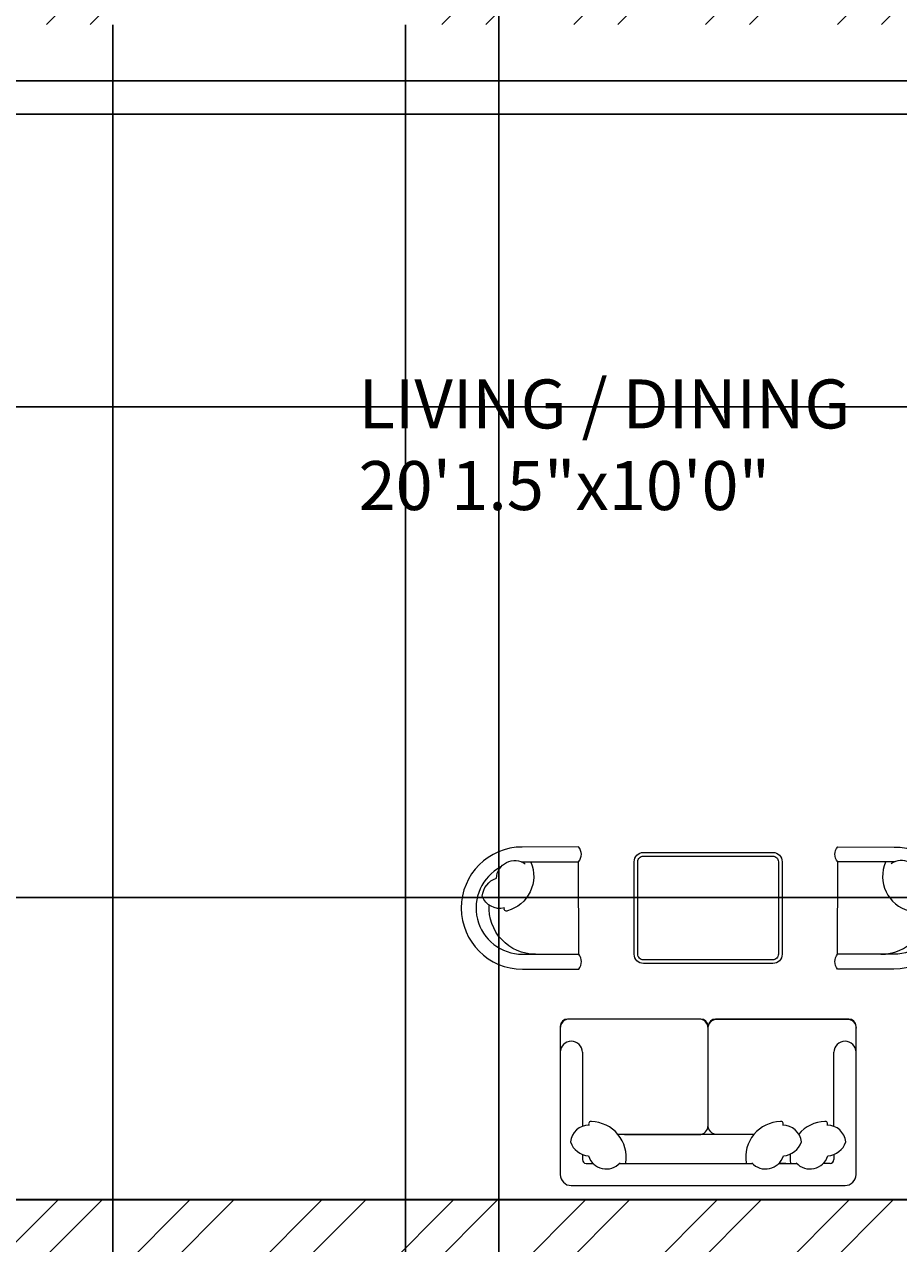
# Model space of a CAD drawing. Units: inches. Extents: x 1748 to 2382, y 1346 to 2284.
# Tile 9 of 26: x 1920 to 2009, y 1730 to 1855. Entities that reach past the tile are written whole.
import ezdxf

# ---------------------------------------------------------------- set-up
doc = ezdxf.new("R2010")
doc.units = ezdxf.units.IN
for name, color, linetype, lineweight in [('A-ANNO-DIMS', 2, 'Continuous', 18), ('A-AREA-IDEN', 7, 'Continuous', 18), ('A-FURN', 8, 'Continuous', 13), ('A-WALL', 7, 'Continuous', 35), ('A-WALL-PATT', 9, 'Continuous', 13)]:
    doc.layers.add(name, color=color, linetype=linetype, lineweight=lineweight)
doc.styles.get("Standard").update_dxf_attribs({"font": 'arial.ttf'})
doc.dimstyles.get("Standard").update_dxf_attribs({"dimtxt": 0.18, "dimasz": 0.18, "dimexe": 0.18, "dimexo": 0.0625, "dimgap": 0.09, "dimtad": 0, "dimtih": 1, "dimtoh": 1, "dimdec": 4, "dimzin": 0, "dimdsep": 46, "dimtxsty": 'Standard', "dimcen": 0.09, "dimadec": 0, "dimazin": 0, "dimtfac": 1, "dimtdec": 4, "dimtofl": 0, "dimtmove": 0, "dimatfit": 3, "dimfxl": 1, "dimtolj": 1, "dimtzin": 0, "dimarcsym": 0})

# ---------------------------------------------------------------- blocks, each defined once
blk = doc.blocks.new('A$C1352')
at = {"color": 0}
for points in [[(0.0027, 0.053), (0.0027, 0.553, -0.414214), (0.0527, 0.603), (0.7527, 0.603, -0.414214), (0.8027, 0.553), (0.8027, 0.053, -0.414214), (0.7527, 0.003), (0.0527, 0.003, -0.414214)], [(0.0227, 0.053), (0.0227, 0.553, -0.414214), (0.0527, 0.583), (0.7527, 0.583, -0.414214), (0.7827, 0.553), (0.7827, 0.053, -0.414214), (0.7527, 0.023), (0.0527, 0.023, -0.414214)]]:
    blk.add_lwpolyline(points, format="xyb", close=True, dxfattribs=at)
blk = doc.blocks.new('CHAIR-LOUNGE')
blk.add_line((1.52, 6.05), (1.51, 0.29))
at = {"ltscale": 0.03}
blk.add_lwpolyline([(1.51, 0.29, -0.369229), (0, 0.29), (0.01, 6.05, -1), (12.48, 6.04), (12.47, 0.28, -0.369229), (10.96, 0.28)], format="xyb", close=True, dxfattribs=at)
blk.add_lwpolyline([(2.05, 8.23, -0.785087), (10.96, 6.04), (10.96, 0.28)], format="xyb")
for centre, radius, start, end in [((5.21, 8.01), 2.13, 94.9999, 161.3534), ((4.35, 8.32), 1.94, 346.6403, 69.4695), ((6.24, 4.71), 4.72, 359.9461, 93.658), ((3.29, 6.8), 1.89, 92.9922, 214.1401), ((3, 8.54), 3.66, 247.0143, 344.2857), ((6.33, 7.66), 0.226, 330.6238, 113.7423), ((6.24, 6.05), 4.72, 178.8536, 179.9461)]:
    blk.add_arc(centre, radius, start, end)
blk = doc.blocks.new('*D48')
at = {"layer": 'A-ANNO-DIMS', "color": 0, "lineweight": -2, "transparency": 16777216}
for p, q in [((2130.9, 1849.07), (1779.88, 1849.07)), ((1780.06, 1848.89), (1780.06, 1832.62)), ((1780.06, 1815.98), (1780.06, 1832.25)), ((2130.9, 1815.8), (1779.88, 1815.8))]:
    blk.add_line(p, q, dxfattribs=at)
at = {"layer": 'A-ANNO-DIMS', "color": 0, "transparency": 16777216}
for points in [[(1780.03, 1848.89), (1780.09, 1848.89), (1780.06, 1849.07)], [(1780.03, 1815.98), (1780.09, 1815.98), (1780.06, 1815.8)]]:
    blk.add_solid(points, dxfattribs=at)
at = {"layer": 'Defpoints', "color": 0, "transparency": 16777216}
for p in [(1780.06, 1849.07), (2130.96, 1849.07), (2130.96, 1815.8)]:
    blk.add_point(p, dxfattribs=at)
at = {"layer": 'A-ANNO-DIMS', "color": 0, "transparency": 16777216, "insert": (1780.06, 1832.43), "char_height": 0.18, "attachment_point": 5}
blk.add_mtext('\\A1;33.27', dxfattribs=at)
blk = doc.blocks.new('*D51')
at = {"layer": 'A-ANNO-DIMS', "color": 0, "lineweight": -2, "transparency": 16777216}
for p, q in [((1968.44, 2223.79), (1968.44, 1360.47)), ((2040.07, 2223.79), (2040.07, 1360.47)), ((1968.62, 1360.65), (2003.86, 1360.65)), ((2039.89, 1360.65), (2004.65, 1360.65))]:
    blk.add_line(p, q, dxfattribs=at)
at = {"layer": 'A-ANNO-DIMS', "color": 0, "transparency": 16777216}
for points in [[(1968.62, 1360.68), (1968.62, 1360.62), (1968.44, 1360.65)], [(2039.89, 1360.68), (2039.89, 1360.62), (2040.07, 1360.65)]]:
    blk.add_solid(points, dxfattribs=at)
at = {"layer": 'Defpoints', "color": 0, "transparency": 16777216}
for p in [(1968.44, 2223.85), (2040.07, 2223.85), (2040.07, 1360.65)]:
    blk.add_point(p, dxfattribs=at)
at = {"layer": 'A-ANNO-DIMS', "color": 0, "transparency": 16777216, "insert": (2004.26, 1360.65), "char_height": 0.18, "attachment_point": 5}
blk.add_mtext('\\A1;71.62', dxfattribs=at)
blk = doc.blocks.new('*D60')
at = {"layer": 'A-ANNO-DIMS', "color": 0, "lineweight": -2, "transparency": 16777216}
for p, q in [((2206.01, 1845.68), (1779.88, 1845.68)), ((1780.06, 1845.5), (1780.06, 1805.86)), ((1780.06, 1765.86), (1780.06, 1805.5)), ((2206.01, 1765.68), (1779.88, 1765.68))]:
    blk.add_line(p, q, dxfattribs=at)
at = {"layer": 'A-ANNO-DIMS', "color": 0, "transparency": 16777216}
for points in [[(1780.03, 1845.5), (1780.09, 1845.5), (1780.06, 1845.68)], [(1780.03, 1765.86), (1780.09, 1765.86), (1780.06, 1765.68)]]:
    blk.add_solid(points, dxfattribs=at)
at = {"layer": 'Defpoints', "color": 0, "transparency": 16777216}
for p in [(1780.06, 1845.68), (2206.07, 1845.68), (2206.07, 1765.68)]:
    blk.add_point(p, dxfattribs=at)
at = {"layer": 'A-ANNO-DIMS', "color": 0, "transparency": 16777216, "insert": (1780.06, 1805.68), "char_height": 0.18, "attachment_point": 5}
blk.add_mtext('\\A1;80', dxfattribs=at)
blk = doc.blocks.new('*D79')
at = {"layer": 'A-ANNO-DIMS', "color": 0, "lineweight": -2, "transparency": 16777216}
for p, q in [((1929, 1854.79), (1929, 1360.47)), ((1958.9, 1854.79), (1958.9, 1360.47)), ((1929.18, 1360.65), (1943.62, 1360.65)), ((1958.72, 1360.65), (1944.27, 1360.65))]:
    blk.add_line(p, q, dxfattribs=at)
at = {"layer": 'A-ANNO-DIMS', "color": 0, "transparency": 16777216}
for points in [[(1929.18, 1360.68), (1929.18, 1360.62), (1929, 1360.65)], [(1958.72, 1360.68), (1958.72, 1360.62), (1958.9, 1360.65)]]:
    blk.add_solid(points, dxfattribs=at)
at = {"layer": 'Defpoints', "color": 0, "transparency": 16777216}
for p in [(1929, 1854.85), (1958.9, 1854.85), (1958.9, 1360.65)]:
    blk.add_point(p, dxfattribs=at)
at = {"layer": 'A-ANNO-DIMS', "color": 0, "transparency": 16777216, "insert": (1943.95, 1360.65), "char_height": 0.18, "attachment_point": 5}
blk.add_mtext('\\A1;29.9', dxfattribs=at)

msp = doc.modelspace()

# ---------------------------------------------------------------- hatches: boundary and pattern name
at = {"layer": 'A-WALL-PATT'}
h = msp.add_hatch(dxfattribs=at)
h.set_pattern_fill('ANSI32', color=256)
h.paths.add_polyline_path([(1908.4445, 2232.8497), (1821.9607, 2232.8497), (1821.9607, 2223.8497), (1865.4607, 2223.8497), (1865.4607, 2209.9185), (1869.9607, 2209.9185), (1869.9607, 2223.8497), (1908.4445, 2223.8497), (1908.4445, 2228.3497)])
h.paths.add_polyline_path([(2040.0683, 2232.8497), (1968.4445, 2232.8497), (1968.4445, 2223.8497), (2025.9607, 2223.8497), (2025.9607, 2130.3497), (2032.1341, 2130.3497), (2032.1341, 2132.5997), (2032.1341, 2134.8497), (2030.4607, 2134.8497), (2030.4607, 2223.8497), (2040.0683, 2223.8497)])
h.paths.add_polyline_path([(2091.3969, 2232.8497), (2064.0683, 2232.8497), (2064.0683, 2223.8497), (2078.4607, 2223.8497), (2078.4607, 2134.8497), (2051.1563, 2134.8497), (2051.1563, 2130.3497), (2078.4607, 2130.3497), (2078.4607, 2128.6813), (2082.9607, 2128.6813), (2082.9607, 2130.3497), (2086.1879, 2130.3497), (2086.1879, 2132.5997), (2086.1879, 2134.8497), (2082.9607, 2134.8497), (2082.9607, 2223.8497), (2091.3969, 2223.8497), (2091.3969, 2228.3497)])
h.paths.add_polyline_path([(2167.0164, 2232.8497), (2115.3969, 2232.8497), (2115.3969, 2223.8497), (2130.9607, 2223.8497), (2130.9607, 2134.8497), (2106.9607, 2134.8497), (2106.9607, 2130.3497), (2135.4607, 2130.3497), (2135.4607, 2223.8497), (2167.0164, 2223.8497), (2167.0164, 2228.3497)])
h.paths.add_polyline_path([(1869.9607, 2149.9185), (1865.4607, 2149.9185), (1865.4607, 2127.8942), (1869.9607, 2127.8942)])
h.paths.add_polyline_path([(2082.9607, 2104.4871), (2080.7107, 2104.4871), (2078.4607, 2104.4871), (2078.4607, 2103.8497), (1869.9607, 2103.8497), (1869.9607, 2108.6062), (1867.7107, 2108.6062), (1865.4607, 2108.6062), (1865.4607, 2103.8497), (1821.9607, 2103.8497), (1821.9607, 2099.3497), (1865.4607, 2099.3497), (1865.4607, 2094.7509), (1869.9607, 2094.7509), (1869.9607, 2099.3497), (2025.9607, 2099.3497), (2025.9607, 2096.4326), (2030.4607, 2096.4326), (2030.4607, 2099.3497), (2082.9607, 2099.3497)])
h.paths.add_polyline_path([(1928.9457, 1401.1212), (2176.8693, 1401.1212), (2176.8693, 1438.214), (1928.9457, 1438.214)], flags=9)
h.paths.add_polyline_path([(2122.2668, 2048.1927), (2177.9387, 2048.1927), (2177.9387, 2066.85), (2122.2668, 2066.85)], flags=9)
h.paths.add_polyline_path([(2272.688, 2153.8197), (2272.688, 2216.746), (2262.3845, 2216.746), (2262.3845, 2153.8197)], flags=9)
h.paths.add_polyline_path([(2157.2928, 2166.5593), (2196.3822, 2166.5593), (2196.3822, 2185.2167), (2157.2928, 2185.2167)], flags=9)
h.paths.add_polyline_path([(2089.3407, 2162.0698), (2124.3987, 2162.0698), (2124.3987, 2180.7272), (2089.3407, 2180.7272)], flags=9)
h.paths.add_polyline_path([(2037.4521, 2160.0913), (2072.5101, 2160.0913), (2072.5101, 2178.7486), (2037.4521, 2178.7486)], flags=9)
h.paths.add_polyline_path([(1884.7894, 2104.1554), (1923.6297, 2104.1554), (1923.6297, 2122.8127), (1884.7894, 2122.8127)], flags=9)
h.paths.add_polyline_path([(1851.2832, 2142.9749), (1851.2832, 2199.3051), (1840.9796, 2199.3051), (1840.9796, 2142.9749)], flags=9)
h.paths.add_polyline_path([(1844.8763, 2017.2834), (1844.8763, 2073.6136), (1834.5728, 2073.6136), (1834.5728, 2017.2834)], flags=9)
h.paths.add_polyline_path([(1897.1577, 2073.1279), (1935.9981, 2073.1279), (1935.9981, 2091.7853), (1897.1577, 2091.7853)], flags=9)
h.paths.add_polyline_path([(1952.3395, 1802.4231), (2008.0114, 1802.4231), (2008.0114, 1821.0805), (1952.3395, 1821.0805)], flags=9)
h.paths.add_polyline_path([(1978.8184, 1857.6841), (2017.7338, 1857.6841), (2017.7338, 1876.3415), (1978.8184, 1876.3415)], flags=9)
h.paths.add_polyline_path([(1979.6513, 1925.9516), (2008.8089, 1925.9516), (2008.8089, 1944.6089), (1979.6513, 1944.6089)], flags=9)
h.paths.add_polyline_path([(1838.5553, 1860.3527), (1877.3957, 1860.3527), (1877.3957, 1879.01), (1838.5553, 1879.01)], flags=9)
h.paths.add_polyline_path([(1883.9018, 1787.3013), (1883.9018, 1843.6315), (1873.5983, 1843.6315), (1873.5983, 1787.3013)], flags=9)
h.paths.add_polyline_path([(1873.7079, 1509.1938), (1873.7079, 1583.7709), (1863.4044, 1583.7709), (1863.4044, 1509.1938)], flags=9)
h.paths.add_polyline_path([(1916.2259, 1603.3681), (1955.0663, 1603.3681), (1955.0663, 1622.0254), (1916.2259, 1622.0254)], flags=9)
h.paths.add_polyline_path([(1876.3013, 1636.757), (1876.3013, 1693.0871), (1865.9978, 1693.0871), (1865.9978, 1636.757)], flags=9)
h.paths.add_polyline_path([(1921.3138, 1521.8316), (1964.0662, 1521.8316), (1964.0662, 1540.489), (1921.3138, 1540.489)], flags=9)
h.paths.add_polyline_path([(2017.5657, 1497.5078), (2046.7983, 1497.5078), (2046.7983, 1516.1651), (2017.5657, 1516.1651)], flags=9)
h.paths.add_polyline_path([(2066.8661, 1499.3902), (2096.0988, 1499.3902), (2096.0988, 1518.0475), (2066.8661, 1518.0475)], flags=9)
h.paths.add_polyline_path([(2155.4835, 1571.6596), (2198.2358, 1571.6596), (2198.2358, 1590.3169), (2155.4835, 1590.3169)], flags=9)
h.paths.add_polyline_path([(2094.9136, 1664.6812), (2150.5855, 1664.6812), (2150.5855, 1683.3386), (2094.9136, 1683.3386)], flags=9)
h.paths.add_polyline_path([(2257.6902, 1863.1628), (2269.8935, 1863.1628), (2269.8935, 1873.4664), (2257.6902, 1873.4664)], flags=9)
h.paths.add_polyline_path([(2164.0748, 1880.3089), (2189.8694, 1880.3089), (2189.8694, 1890.6124), (2164.0748, 1890.6124)], flags=9)
h.paths.add_polyline_path([(2239.4394, 1931.0585), (2268.8187, 1931.0585), (2268.8187, 1949.7159), (2239.4394, 1949.7159)], flags=9)
h = msp.add_hatch(dxfattribs=at)
h.set_pattern_fill('ANSI32', color=256)
h.paths.add_polyline_path([(2297.4607, 2232.8497), (2203.0164, 2232.8497), (2203.0164, 2223.8497), (2244.9607, 2223.8497), (2244.9607, 2127.8554), (2249.4607, 2127.8554), (2249.4607, 2223.8497), (2297.4607, 2223.8497)])
h.paths.add_polyline_path([(2297.4607, 2103.8497), (2249.4607, 2103.8497), (2249.4607, 2106.7497), (2247.2107, 2106.7497), (2244.9607, 2106.7497), (2244.9607, 2103.8497), (2130.9607, 2103.8497), (2130.9607, 2099.3497), (2288.4607, 2099.3497), (2288.4607, 2077.2008), (2297.4607, 2077.2008)])
h.paths.add_polyline_path([(1928.9457, 1401.1212), (2176.8693, 1401.1212), (2176.8693, 1438.214), (1928.9457, 1438.214)], flags=9)
h.paths.add_polyline_path([(2122.2668, 2048.1927), (2177.9387, 2048.1927), (2177.9387, 2066.85), (2122.2668, 2066.85)], flags=9)
h.paths.add_polyline_path([(2272.688, 2153.8197), (2272.688, 2216.746), (2262.3845, 2216.746), (2262.3845, 2153.8197)], flags=25)
h.paths.add_polyline_path([(2157.2928, 2166.5593), (2196.3822, 2166.5593), (2196.3822, 2185.2167), (2157.2928, 2185.2167)], flags=9)
h.paths.add_polyline_path([(2089.3407, 2162.0698), (2124.3987, 2162.0698), (2124.3987, 2180.7272), (2089.3407, 2180.7272)], flags=9)
h.paths.add_polyline_path([(2037.4521, 2160.0913), (2072.5101, 2160.0913), (2072.5101, 2178.7486), (2037.4521, 2178.7486)], flags=9)
h.paths.add_polyline_path([(1884.7894, 2104.1554), (1923.6297, 2104.1554), (1923.6297, 2122.8127), (1884.7894, 2122.8127)], flags=9)
h.paths.add_polyline_path([(1851.2832, 2142.9749), (1851.2832, 2199.3051), (1840.9796, 2199.3051), (1840.9796, 2142.9749)], flags=9)
h.paths.add_polyline_path([(1844.8763, 2017.2834), (1844.8763, 2073.6136), (1834.5728, 2073.6136), (1834.5728, 2017.2834)], flags=9)
h.paths.add_polyline_path([(1897.1577, 2073.1279), (1935.9981, 2073.1279), (1935.9981, 2091.7853), (1897.1577, 2091.7853)], flags=9)
h.paths.add_polyline_path([(1952.3395, 1802.4231), (2008.0114, 1802.4231), (2008.0114, 1821.0805), (1952.3395, 1821.0805)], flags=9)
h.paths.add_polyline_path([(1978.8184, 1857.6841), (2017.7338, 1857.6841), (2017.7338, 1876.3415), (1978.8184, 1876.3415)], flags=9)
h.paths.add_polyline_path([(1979.6513, 1925.9516), (2008.8089, 1925.9516), (2008.8089, 1944.6089), (1979.6513, 1944.6089)], flags=9)
h.paths.add_polyline_path([(1838.5553, 1860.3527), (1877.3957, 1860.3527), (1877.3957, 1879.01), (1838.5553, 1879.01)], flags=9)
h.paths.add_polyline_path([(1883.9018, 1787.3013), (1883.9018, 1843.6315), (1873.5983, 1843.6315), (1873.5983, 1787.3013)], flags=9)
h.paths.add_polyline_path([(1873.7079, 1509.1938), (1873.7079, 1583.7709), (1863.4044, 1583.7709), (1863.4044, 1509.1938)], flags=9)
h.paths.add_polyline_path([(1916.2259, 1603.3681), (1955.0663, 1603.3681), (1955.0663, 1622.0254), (1916.2259, 1622.0254)], flags=9)
h.paths.add_polyline_path([(1876.3013, 1636.757), (1876.3013, 1693.0871), (1865.9978, 1693.0871), (1865.9978, 1636.757)], flags=9)
h.paths.add_polyline_path([(1921.3138, 1521.8316), (1964.0662, 1521.8316), (1964.0662, 1540.489), (1921.3138, 1540.489)], flags=9)
h.paths.add_polyline_path([(2017.5657, 1497.5078), (2046.7983, 1497.5078), (2046.7983, 1516.1651), (2017.5657, 1516.1651)], flags=9)
h.paths.add_polyline_path([(2066.8661, 1499.3902), (2096.0988, 1499.3902), (2096.0988, 1518.0475), (2066.8661, 1518.0475)], flags=9)
h.paths.add_polyline_path([(2155.4835, 1571.6596), (2198.2358, 1571.6596), (2198.2358, 1590.3169), (2155.4835, 1590.3169)], flags=9)
h.paths.add_polyline_path([(2094.9136, 1664.6812), (2150.5855, 1664.6812), (2150.5855, 1683.3386), (2094.9136, 1683.3386)], flags=9)
h.paths.add_polyline_path([(2257.6902, 1863.1628), (2269.8935, 1863.1628), (2269.8935, 1873.4664), (2257.6902, 1873.4664)], flags=9)
h.paths.add_polyline_path([(2164.0748, 1880.3089), (2189.8694, 1880.3089), (2189.8694, 1890.6124), (2164.0748, 1890.6124)], flags=9)
h.paths.add_polyline_path([(2239.4394, 1931.0585), (2268.8187, 1931.0585), (2268.8187, 1949.7159), (2239.4394, 1949.7159)], flags=9)
h = msp.add_hatch(dxfattribs=at)
h.set_pattern_fill('ANSI32', color=256)
h.paths.add_polyline_path([(1919.6777, 1476.8497), (1900.6426, 1476.8497), (1900.6426, 1522.0826), (1898.3926, 1522.0826), (1896.1426, 1522.0826), (1896.1426, 1476.8497), (1857.1426, 1476.8497), (1857.1426, 1467.8497), (1896.1426, 1467.8497), (1919.6777, 1467.8497), (1919.6777, 1472.3497)])
h.paths.add_polyline_path([(2018.7873, 1472.3497), (2018.7873, 1476.8497), (2010.9607, 1476.8497), (2010.9607, 1560.8497), (2034.9607, 1560.8497), (2034.9607, 1565.3497), (2006.4607, 1565.3497), (2006.4607, 1476.8497), (1955.6777, 1476.8497), (1955.6777, 1467.8497), (2018.7873, 1467.8497)])
h.paths.add_polyline_path([(2152.3354, 1472.3497), (2152.3354, 1476.8497), (2115.9607, 1476.8497), (2115.9607, 1565.3497), (2109.2204, 1565.3497), (2109.2204, 1563.0997), (2109.2204, 1560.8497), (2111.4607, 1560.8497), (2111.4607, 1476.8497), (2095.3617, 1476.8497), (2095.3617, 1467.8497), (2152.3354, 1467.8497)])
h.paths.add_polyline_path([(2071.3617, 1476.8497), (2063.4607, 1476.8497), (2063.4607, 1560.8497), (2090.1865, 1560.8497), (2090.1865, 1565.3497), (2063.4607, 1565.3497), (2063.4607, 1572.5485), (2061.2107, 1572.5485), (2058.9607, 1572.5485), (2058.9607, 1565.3497), (2055.6281, 1565.3497), (2055.6281, 1560.8497), (2058.9607, 1560.8497), (2058.9607, 1476.8497), (2042.7873, 1476.8497), (2042.7873, 1467.8497), (2071.3617, 1467.8497), (2071.3617, 1472.3497)])
h.paths.add_polyline_path([(2297.4607, 1506.5652), (2288.4607, 1506.5652), (2288.4607, 1476.8497), (2212.3354, 1476.8497), (2212.3354, 1467.8497), (2297.4607, 1467.8497)])
h.paths.add_polyline_path([(2297.4607, 1645.3038), (2288.4607, 1645.3038), (2288.4607, 1605.8497), (2058.9607, 1605.8497), (2058.9607, 1600.1857), (2061.2107, 1600.1857), (2063.4607, 1600.1857), (2063.4607, 1601.3497), (2288.4607, 1601.3497), (2288.4607, 1566.5652), (2297.4607, 1566.5652)])
h.paths.add_polyline_path([(2010.9607, 1609.0561), (2008.7107, 1609.0561), (2006.4607, 1609.0561), (2006.4607, 1605.8497), (1900.6426, 1605.8497), (1900.6426, 1609.7171), (1898.3926, 1609.7171), (1896.1426, 1609.7171), (1896.1426, 1605.8497), (1857.1426, 1605.8497), (1857.1426, 1601.3497), (1896.1426, 1601.3497), (1896.1426, 1542.5447), (1900.6426, 1542.5447), (1900.6426, 1601.3497), (2010.9607, 1601.3497)])
h.paths.add_polyline_path([(1928.9457, 1401.1212), (2176.8693, 1401.1212), (2176.8693, 1438.214), (1928.9457, 1438.214)], flags=9)
h.paths.add_polyline_path([(2122.2668, 2048.1927), (2177.9387, 2048.1927), (2177.9387, 2066.85), (2122.2668, 2066.85)], flags=9)
h.paths.add_polyline_path([(2272.688, 2153.8197), (2272.688, 2216.746), (2262.3845, 2216.746), (2262.3845, 2153.8197)], flags=9)
h.paths.add_polyline_path([(2157.2928, 2166.5593), (2196.3822, 2166.5593), (2196.3822, 2185.2167), (2157.2928, 2185.2167)], flags=9)
h.paths.add_polyline_path([(2089.3407, 2162.0698), (2124.3987, 2162.0698), (2124.3987, 2180.7272), (2089.3407, 2180.7272)], flags=9)
h.paths.add_polyline_path([(2037.4521, 2160.0913), (2072.5101, 2160.0913), (2072.5101, 2178.7486), (2037.4521, 2178.7486)], flags=9)
h.paths.add_polyline_path([(1884.7894, 2104.1554), (1923.6297, 2104.1554), (1923.6297, 2122.8127), (1884.7894, 2122.8127)], flags=9)
h.paths.add_polyline_path([(1851.2832, 2142.9749), (1851.2832, 2199.3051), (1840.9796, 2199.3051), (1840.9796, 2142.9749)], flags=9)
h.paths.add_polyline_path([(1844.8763, 2017.2834), (1844.8763, 2073.6136), (1834.5728, 2073.6136), (1834.5728, 2017.2834)], flags=9)
h.paths.add_polyline_path([(1897.1577, 2073.1279), (1935.9981, 2073.1279), (1935.9981, 2091.7853), (1897.1577, 2091.7853)], flags=9)
h.paths.add_polyline_path([(1952.3395, 1802.4231), (2008.0114, 1802.4231), (2008.0114, 1821.0805), (1952.3395, 1821.0805)], flags=9)
h.paths.add_polyline_path([(1978.8184, 1857.6841), (2017.7338, 1857.6841), (2017.7338, 1876.3415), (1978.8184, 1876.3415)], flags=9)
h.paths.add_polyline_path([(1979.6513, 1925.9516), (2008.8089, 1925.9516), (2008.8089, 1944.6089), (1979.6513, 1944.6089)], flags=9)
h.paths.add_polyline_path([(1838.5553, 1860.3527), (1877.3957, 1860.3527), (1877.3957, 1879.01), (1838.5553, 1879.01)], flags=9)
h.paths.add_polyline_path([(1883.9018, 1787.3013), (1883.9018, 1843.6315), (1873.5983, 1843.6315), (1873.5983, 1787.3013)], flags=9)
h.paths.add_polyline_path([(1873.7079, 1509.1938), (1873.7079, 1583.7709), (1863.4044, 1583.7709), (1863.4044, 1509.1938)], flags=9)
h.paths.add_polyline_path([(1916.2259, 1603.3681), (1955.0663, 1603.3681), (1955.0663, 1622.0254), (1916.2259, 1622.0254)], flags=9)
h.paths.add_polyline_path([(1876.3013, 1636.757), (1876.3013, 1693.0871), (1865.9978, 1693.0871), (1865.9978, 1636.757)], flags=9)
h.paths.add_polyline_path([(1921.3138, 1521.8316), (1964.0662, 1521.8316), (1964.0662, 1540.489), (1921.3138, 1540.489)], flags=9)
h.paths.add_polyline_path([(2017.5657, 1497.5078), (2046.7983, 1497.5078), (2046.7983, 1516.1651), (2017.5657, 1516.1651)], flags=9)
h.paths.add_polyline_path([(2066.8661, 1499.3902), (2096.0988, 1499.3902), (2096.0988, 1518.0475), (2066.8661, 1518.0475)], flags=9)
h.paths.add_polyline_path([(2155.4835, 1571.6596), (2198.2358, 1571.6596), (2198.2358, 1590.3169), (2155.4835, 1590.3169)], flags=25)
h.paths.add_polyline_path([(2094.9136, 1664.6812), (2150.5855, 1664.6812), (2150.5855, 1683.3386), (2094.9136, 1683.3386)], flags=9)
h.paths.add_polyline_path([(2257.6902, 1863.1628), (2269.8935, 1863.1628), (2269.8935, 1873.4664), (2257.6902, 1873.4664)], flags=9)
h.paths.add_polyline_path([(2164.0748, 1880.3089), (2189.8694, 1880.3089), (2189.8694, 1890.6124), (2164.0748, 1890.6124)], flags=9)
h.paths.add_polyline_path([(2239.4394, 1931.0585), (2268.8187, 1931.0585), (2268.8187, 1949.7159), (2239.4394, 1949.7159)], flags=9)
h = msp.add_hatch(dxfattribs=at)
h.set_pattern_fill('ANSI32', color=256)
h.paths.add_polyline_path([(1900.6426, 1652.723), (1896.1426, 1652.723), (1896.1426, 1629.9029), (1900.6426, 1629.9029)])
h.paths.add_polyline_path([(2206.0699, 1859.3497), (2197.0699, 1859.3497), (2197.0699, 1734.8497), (2206.0699, 1734.8497)], flags=17)
h.paths.add_polyline_path([(2297.4607, 1865.3269), (2288.4607, 1865.3269), (2288.4607, 1734.8497), (2206.0699, 1734.8497), (2180.4551, 1734.8497), (2180.4551, 1725.8497), (2197.0699, 1725.8497), (2206.0699, 1725.8497), (2288.4607, 1725.8497), (2288.4607, 1705.3038), (2297.4607, 1705.3038)])
h.paths.add_polyline_path([(2139.9607, 1815.8001), (2135.4607, 1815.8001), (2130.9607, 1815.8001), (2130.9607, 1734.8497), (1900.6426, 1734.8497), (1900.6426, 1738.9477), (1898.3926, 1738.9477), (1896.1426, 1738.9477), (1896.1426, 1734.8497), (1857.1426, 1734.8497), (1857.1426, 1725.8497), (1896.1426, 1725.8497), (1896.1426, 1712.723), (1900.6426, 1712.723), (1900.6426, 1725.8497), (2006.4607, 1725.8497), (2006.4607, 1637.448), (2010.9607, 1637.448), (2010.9607, 1725.8497), (2139.9607, 1725.8497), (2147.389, 1725.8497), (2147.389, 1730.3497), (2147.389, 1734.8497), (2139.9607, 1734.8497)])
h.paths.add_polyline_path([(2149.8497, 1917.8497), (2149.8497, 1922.3497), (2139.9607, 1922.3497), (2139.9607, 1979.3497), (2030.4607, 1979.3497), (2030.4607, 2069.8971), (2028.2107, 2069.8971), (2025.9607, 2069.8971), (2025.9607, 1979.3497), (1869.9607, 1979.3497), (1869.9607, 1998.93), (1865.4607, 1998.93), (1865.4607, 1979.3497), (1821.9607, 1979.3497), (1821.9607, 1952.7922), (1826.9306, 1952.7922), (1830.9607, 1952.7922), (1830.9607, 1970.3497), (1962.9607, 1970.3497), (1962.9607, 1926.5713), (1967.4607, 1926.5713), (1967.4607, 1970.3497), (2027.4607, 1970.3497), (2027.4607, 1898.3497), (2004.9604, 1898.3497), (2004.9604, 1893.8497), (2027.4607, 1893.8497), (2027.4607, 1859.3497), (1958.8973, 1859.3497), (1958.8973, 1854.8497), (2047.917, 1854.8497), (2047.917, 1859.3497), (2031.9607, 1859.3497), (2031.9607, 1970.3497), (2130.9607, 1970.3497), (2130.9607, 1859.3497), (2104.9565, 1859.3497), (2104.9565, 1854.8497), (2130.9607, 1854.8497), (2130.9607, 1849.0684), (2139.9607, 1849.0684), (2139.9607, 1913.3497), (2149.8497, 1913.3497)])
h.paths.add_polyline_path([(1928.9996, 1859.3497), (1830.9607, 1859.3497), (1830.9607, 1892.7922), (1821.9607, 1892.7922), (1821.9607, 1854.8497), (1896.1426, 1854.8497), (1896.1426, 1836.6443), (1898.378, 1836.6443), (1900.6426, 1836.6443), (1900.6426, 1854.8497), (1928.9996, 1854.8497), (1928.9996, 1857.0997)])
h.paths.add_polyline_path([(1980.9604, 1896.0997), (1980.9604, 1898.3497), (1967.4607, 1898.3497), (1967.4607, 1902.3846), (1962.9607, 1902.3846), (1962.9607, 1859.3497), (1967.4607, 1859.3497), (1967.4607, 1893.8497), (1980.9604, 1893.8497)], flags=17)
h.paths.add_polyline_path([(1900.6426, 1776.6443), (1896.1426, 1776.6443), (1896.1426, 1758.0891), (1900.6426, 1758.0891)], flags=17)
h.paths.add_polyline_path([(2297.4607, 2017.2008), (2288.4607, 2017.2008), (2288.4607, 1979.3497), (2213.4607, 1979.3497), (2213.4607, 1922.3497), (2183.3516, 1922.3497), (2183.3516, 1913.3497), (2213.4607, 1913.3497), (2236.234, 1913.3497), (2236.234, 1922.3497), (2222.4607, 1922.3497), (2222.4607, 1931.3497), (2222.4607, 1970.3497), (2288.4607, 1970.3497), (2288.4607, 1922.3497), (2272.1921, 1922.3497), (2272.1921, 1913.3497), (2288.4607, 1913.3497), (2288.4607, 1901.3269), (2297.4607, 1901.3269)])

# ---------------------------------------------------------------- linework, layer by layer
at = {"layer": 'A-FURN'}
for p, q in [((1976.966, 1749.8844), (1976.966, 1742.3196)), ((2002.6636, 1742.3196), (2002.6636, 1749.8844)), ((1976.966, 1739.4513), (1976.966, 1738.9252)), ((2002.6636, 1739.4513), (2002.6636, 1738.9252)), ((1977.3439, 1738.5472), (1978.0391, 1738.5472)), ((1980.7673, 1738.5472), (1994.3258, 1738.5472)), ((1997.7491, 1738.5472), (1997.0539, 1738.5472)), ((1997.0539, 1738.5472), (1998.8623, 1738.5472)), ((2002.2857, 1738.5472), (2001.5905, 1738.5472))]:
    msp.add_line(p, q, dxfattribs=at)
at = {"layer": 'A-FURN', "ltscale": 0.03}
msp.add_lwpolyline([(1989.8055, 1752.5298, 0.41421356), (1989.0497, 1753.2856), (1975.4544, 1753.2856, 0.41421356), (1974.6986, 1752.5298), (1974.6986, 1737.4135, 0.41421356), (1975.8323, 1736.2798), (2003.7973, 1736.2798, 0.41421356), (2004.931, 1737.4135), (2004.931, 1752.5298, 0.41421356), (2004.1752, 1753.2856), (1990.5799, 1753.2856, 0.41421356), (1989.8241, 1752.5298)], format="xyb", dxfattribs=at)
at = {"layer": 'A-FURN'}
for points in [[(1981.2591, 1741.476), (1988.8701, 1741.476, 0.41421356), (1989.8148, 1742.4208), (1989.8148, 1752.3408, 0.41421356), (1988.8701, 1753.2856), (1975.6433, 1753.2856, 0.41421356), (1974.6986, 1752.3408)], [(1994.4774, 1741.476), (1990.7596, 1741.476, -0.41421356), (1989.8148, 1742.4208), (1989.8148, 1752.3408, -0.41421356), (1990.7596, 1753.2856), (2003.9863, 1753.2856, -0.41421356), (2004.931, 1752.3408)]]:
    msp.add_lwpolyline(points, format="xyb", dxfattribs=at)
msp.add_lwpolyline([(1994.4774, 1741.476), (1980.6157, 1741.476)], dxfattribs=at)
for centre, radius, start, end in [((1975.8323, 1749.8844), 1.1337, 90, 180), ((1975.8323, 1749.8844), 1.1337, 0, 90), ((2003.7973, 1749.8844), 1.1337, 90, 180), ((2003.7973, 1749.8844), 1.1337, 0, 90), ((1977.6783, 1740.5132), 1.9418, 90.743002, 173.572142), ((1977.8316, 1742.5935), 0.226, 74.72647, 217.845006), ((1977.7883, 1739.155), 3.658, 351.11695, 88.388369), ((1997.3048, 1739.155), 3.658, 91.611631, 188.88305), ((1997.2614, 1742.5935), 0.226, 322.154994, 105.27353), ((1997.4148, 1740.5132), 1.9418, 6.427858, 89.256998), ((2001.8413, 1739.155), 3.658, 91.611631, 139.375991), ((2001.798, 1742.5935), 0.226, 322.154994, 105.27353), ((2001.9513, 1740.5132), 1.9418, 6.427858, 89.256998), ((1977.7624, 1741.428), 2.1311, 199.10261, 265.456062), ((1997.3306, 1741.428), 2.1311, 274.543938, 340.89739), ((2001.8672, 1741.428), 2.1311, 274.543938, 340.89739), ((1979.4032, 1739.8601), 1.8933, 197.094904, 318.242764), ((1995.6898, 1739.8601), 1.8933, 221.757236, 342.905096), ((2001.8413, 1739.155), 3.658, 174.880983, 188.88305), ((2000.2264, 1739.8601), 1.8933, 221.757236, 342.905096), ((1977.3439, 1738.9252), 0.3779, 180, 270), ((2002.2857, 1738.9252), 0.3779, 270, 0), ((2002.2857, 1738.9252), 0.3779, 270, 0)]:
    msp.add_arc(centre, radius, start, end, dxfattribs=at)
at = {"layer": 'A-WALL'}
msp.add_line((1900.6426, 1734.8497), (2130.9607, 1734.8497), dxfattribs=at)

# ---------------------------------------------------------------- block references
at = {"layer": 'A-FURN', "extrusion": (0, 0, -1), "zscale": -1, "rotation": 270}
msp.add_blockref('CHAIR-LOUNGE', (-1976.872, 1770.8585), dxfattribs=at)
at = {"layer": 'A-FURN', "rotation": 270}
msp.add_blockref('CHAIR-LOUNGE', (2002.7577, 1770.8585), dxfattribs=at)
at = {"layer": 'A-FURN', "ltscale": 0.03, "xscale": 18.89529246734385, "yscale": 18.89529246734385, "zscale": 18.89529246734385, "rotation": 180}
msp.add_blockref('A$C1352', (1997.4237, 1770.3479), dxfattribs=at)

# ---------------------------------------------------------------- texts
at = {"layer": 'A-AREA-IDEN', "insert": (1954.1011, 1818.5924), "char_height": 5, "attachment_point": 1}
msp.add_mtext_dynamic_manual_height_columns('LIVING / DINING\\P20\'1.5"x10\'0"', width=119.140935, gutter_width=12.5, heights=[0], dxfattribs=at)

# ---------------------------------------------------------------- dimensions: what is measured, and where the dimension line sits
at = {"layer": 'A-ANNO-DIMS'}
for base, p1, p2, override, picture, middle in [((2040.0683, 1360.6451), (1968.4445, 2223.8497), (2040.0683, 2223.8497), {"dimdec": 2, "dimlfac": 1, "dimrnd": 0, "dimzin": 0, "dimdsep": 46, "dimlunit": 2}, '*D51', (2004.2564, 1360.6451)), ((1958.8973, 1360.6451), (1928.9996, 1854.8497), (1958.8973, 1854.8497), {"dimdec": 1, "dimlfac": 1, "dimrnd": 0, "dimzin": 0, "dimdsep": 46, "dimlunit": 2}, '*D79', (1943.9485, 1360.6451))]:
    dim = msp.add_linear_dim(base=base, p1=p1, p2=p2, dimstyle='Standard', override=override, dxfattribs=at)
    dim.commit()
    dim.dimension.update_dxf_attribs({"geometry": picture, "text_midpoint": middle})
for base, p1, p2, override, picture, middle in [((1780.0607, 1849.0684), (2130.9607, 1815.8001), (2130.9607, 1849.0684), {"dimdec": 2, "dimlfac": 1, "dimrnd": 0, "dimzin": 0, "dimdsep": 46, "dimlunit": 2}, '*D48', (1780.0607, 1832.4343)), ((1780.0607, 1845.6799), (2206.0699, 1765.6799), (2206.0699, 1845.6799), {"dimdec": 0, "dimlfac": 1, "dimrnd": 0, "dimzin": 0, "dimdsep": 46, "dimlunit": 2}, '*D60', (1780.0607, 1805.6799))]:
    dim = msp.add_linear_dim(base=base, p1=p1, p2=p2, angle=90, dimstyle='Standard', override=override, dxfattribs=at)
    dim.commit()
    dim.dimension.update_dxf_attribs({"geometry": picture, "text_midpoint": middle})

doc.saveas('drawing.dxf')
